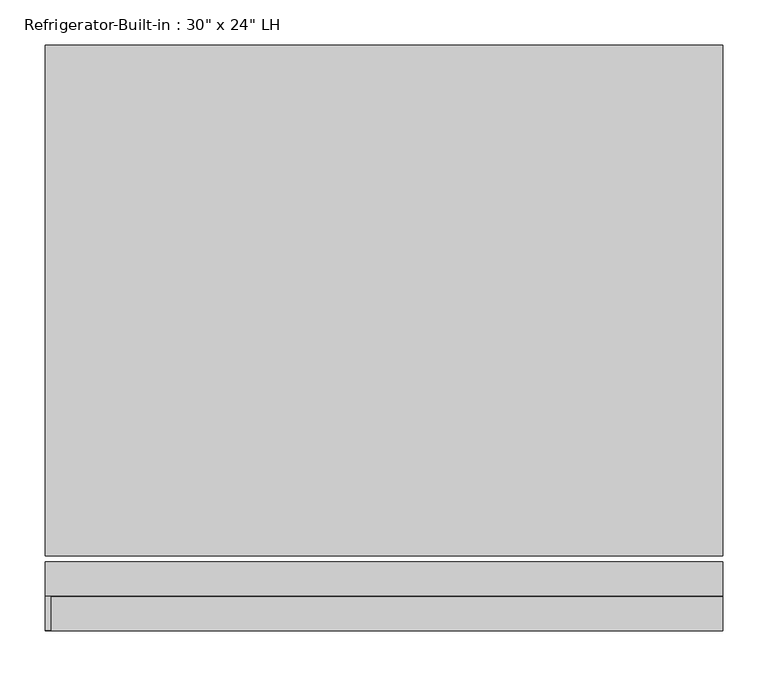
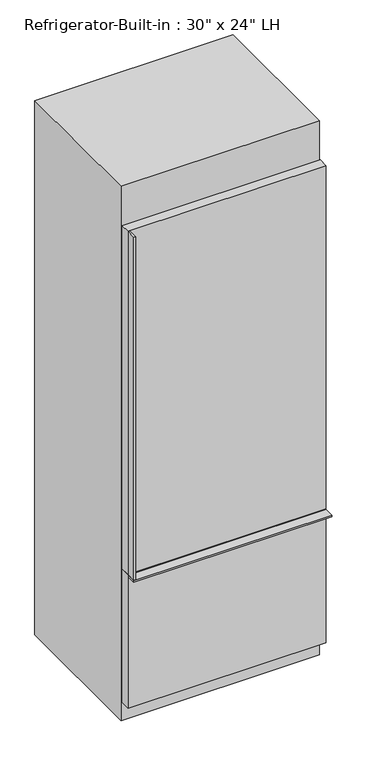
"""IFC4 building model written with IfcOpenShell, lengths in millimetres: proxy geometry."""

from ifc_helpers import new_model, si_unit, frame, origin, origin_with_axes, place, context, project, spatial, polyline, outline, extrude, source, transform, mapped, element, save


def proxy_19935bb1(model_context):
    return source(origin(), model_context, "Body", "SweptSolid", [
        extrude(outline(polyline([(374.65, 290.1239715), (374.65, -275.0260285), (-374.65, -275.0260285), (-374.65, 290.1239715), (374.65, 290.1239715)])), origin_with_axes(), (0.0, 0.0, 1.0), 2133.6),
        extrude(outline(polyline([(374.65, -281.3760285), (374.65, -319.4760285), (-374.65, -319.4760285), (-374.65, -281.3760285), (374.65, -281.3760285)])), frame((0.0, 0.0, 611.1875), z_axis=(0.0, 0.0, 1.0), x_axis=(1.0, 0.0, 0.0)), (0.0, 0.0, 1.0), 1370.0125),
        extrude(outline(polyline([(374.65, -281.3760285), (374.65, -319.4760285), (-374.65, -319.4760285), (-374.65, -281.3760285), (374.65, -281.3760285)])), frame((0.0, 0.0, 76.2), z_axis=(0.0, 0.0, 1.0), x_axis=(1.0, 0.0, 0.0)), (0.0, 0.0, 1.0), 531.8125),
        extrude(outline(polyline([(374.65, -319.4760285), (374.65, -357.5760285), (-374.65, -357.5760285), (-374.65, -319.4760285), (374.65, -319.4760285)])), frame((0.0, 0.0, 601.6625), z_axis=(0.0, 0.0, 1.0), x_axis=(1.0, 0.0, 0.0)), (0.0, 0.0, 1.0), 6.35),
        extrude(outline(polyline([(-374.65, -319.4760285), (-368.3, -319.4760285), (-368.3, -357.5760285), (-374.65, -357.5760285), (-374.65, -319.4760285)])), frame((0.0, 0.0, 611.1875), z_axis=(0.0, 0.0, 1.0), x_axis=(1.0, 0.0, 0.0)), (0.0, 0.0, 1.0), 1370.0125),
    ])


if __name__ == "__main__":
    model = new_model("IFC4")
    model_context = context("Model", 3, world=origin())
    ifc_project = project(units=[si_unit("LENGTHUNIT", "METRE", prefix="MILLI")], contexts=[model_context])
    site = spatial("IfcSite", under=ifc_project)
    building = spatial("IfcBuilding", under=site)
    placement = place(None, origin())
    proxy_shape = proxy_19935bb1(model_context)
    element("IfcBuildingElementProxy", 1, Name="Refrigerator-Built-in : 30\" x 24\" LH", ObjectType="Refrigerator-Built-in : 30\" x 24\" LH", at=placement, inside=building, context=model_context, shape_type="MappedRepresentation", body=[
        mapped(proxy_shape, transform((0.0, 0.0, 0.0), x_axis=(1.0, 0.0, 0.0), y_axis=(0.0, 1.0, 0.0), z_axis=(0.0, 0.0, 1.0))),
    ])
    save(model, "model.ifc")

# Revit data of these elements
# Type "Refrigerator-Built-in : 30\" x 24\" LH"
#   Assembly Code = "E1090400"
#   Depth = 2' - 0"
#   Handle = 0' - 0 1/4"
#   Height = 7' - 0"
#   Top Door Height = 5' - 0"
#   Width = 2' - 5 1/2"
#   Material = Metal - Paint Finish - Ivory,Glossy
#   Default Elevation = 0
# Element 1 (IfcBuildingElementProxy, "Refrigerator-Built-in : 30\" x 24\" LH")
#   Materials on its faces: "Metal - Paint Finish - Ivory,Glossy", "Metal - Chrome"
# Materials
#   "Metal - Paint Finish - Ivory,Glossy": colour RGB 247 247 239, transparency 0
#   "Metal - Chrome": colour RGB 57 57 57, transparency 0
